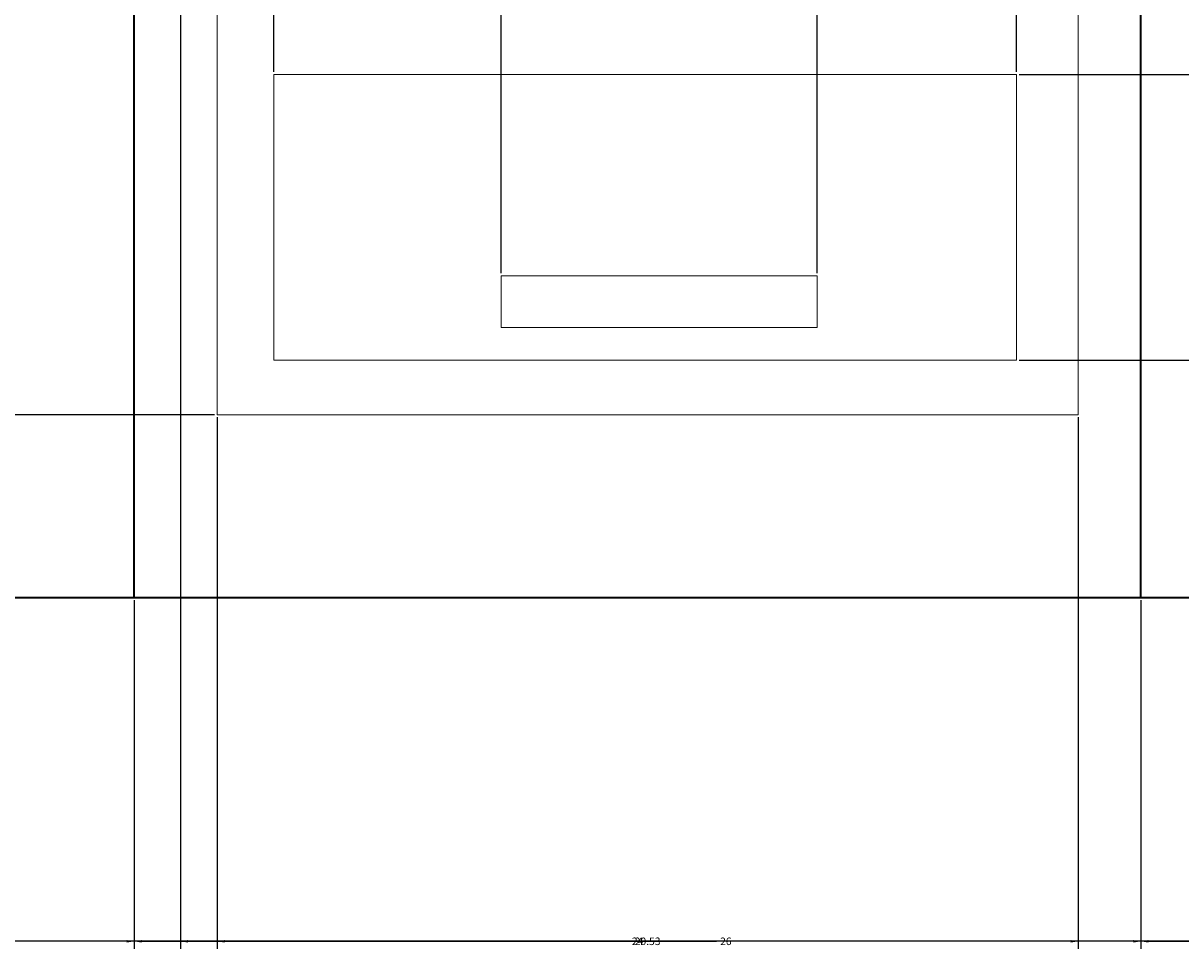
# Model space of a CAD drawing. Units: inches. Extents: x 27 to 200, y -50 to 102.
# Tile 10 of 26: x 117 to 144, y -25 to -3. Entities that reach past the tile are written whole.
import ezdxf

# ---------------------------------------------------------------- set-up
doc = ezdxf.new("R2010")
doc.units = ezdxf.units.IN
doc.header["$MEASUREMENT"] = 0
for name, color, linetype, lineweight in [('A-ANNO-DIMS', 2, 'Continuous', 18), ('A-ELEV', 7, 'Continuous', 35), ('A-FURN', 8, 'Continuous', 18)]:
    doc.layers.add(name, color=color, linetype=linetype, lineweight=lineweight)
doc.styles.get("Standard").update_dxf_attribs({"font": 'arial.ttf'})
doc.dimstyles.get("Standard").update_dxf_attribs({"dimtxt": 0.18, "dimasz": 0.18, "dimexe": 0.18, "dimexo": 0.0625, "dimgap": 0.09, "dimtad": 0, "dimtih": 1, "dimtoh": 1, "dimdec": 4, "dimzin": 0, "dimdsep": 46, "dimtxsty": 'Standard', "dimcen": 0.09, "dimadec": 0, "dimazin": 0, "dimtfac": 1, "dimtdec": 4, "dimtofl": 0, "dimtmove": 0, "dimatfit": 3, "dimfxl": 1, "dimtolj": 1, "dimtzin": 0, "dimarcsym": 0})

# ---------------------------------------------------------------- blocks, each defined once
blk = doc.blocks.new('*D23')
at = {"layer": 'A-ANNO-DIMS', "color": 0, "lineweight": -2, "transparency": 16777216}
for p, q in [((35.417, -16.832), (35.417, -25.149)), ((191.417, -16.832), (191.417, -25.149)), ((35.597, -24.969), (113.137, -24.969)), ((191.237, -24.969), (113.697, -24.969))]:
    blk.add_line(p, q, dxfattribs=at)
at = {"layer": 'A-ANNO-DIMS', "color": 0, "transparency": 16777216}
for points in [[(35.597, -24.939), (35.597, -24.999), (35.417, -24.969)], [(191.237, -24.939), (191.237, -24.999), (191.417, -24.969)]]:
    blk.add_solid(points, dxfattribs=at)
at = {"layer": 'Defpoints', "color": 0, "transparency": 16777216}
for p in [(35.417, -16.769), (191.417, -16.769), (191.417, -24.969)]:
    blk.add_point(p, dxfattribs=at)
at = {"layer": 'A-ANNO-DIMS', "color": 0, "transparency": 16777216, "insert": (113.417, -24.969), "char_height": 0.18, "attachment_point": 5}
blk.add_mtext('\\A1;156', dxfattribs=at)
blk = doc.blocks.new('*D36')
at = {"layer": 'A-ANNO-DIMS', "color": 0, "lineweight": -2, "transparency": 16777216}
for p, q in [((107.312, -16.832), (107.312, -25.149)), ((119.312, -16.832), (119.312, -25.149)), ((107.492, -24.969), (113.102, -24.969)), ((119.132, -24.969), (113.521, -24.969))]:
    blk.add_line(p, q, dxfattribs=at)
at = {"layer": 'A-ANNO-DIMS', "color": 0, "transparency": 16777216}
for points in [[(107.492, -24.939), (107.492, -24.999), (107.312, -24.969)], [(119.132, -24.939), (119.132, -24.999), (119.312, -24.969)]]:
    blk.add_solid(points, dxfattribs=at)
at = {"layer": 'Defpoints', "color": 0, "transparency": 16777216}
for p in [(107.312, -16.769), (119.312, -16.769), (119.312, -24.969)]:
    blk.add_point(p, dxfattribs=at)
at = {"layer": 'A-ANNO-DIMS', "color": 0, "transparency": 16777216, "insert": (113.312, -24.969), "char_height": 0.18, "attachment_point": 5}
blk.add_mtext('\\A1;12', dxfattribs=at)
blk = doc.blocks.new('*D37')
at = {"layer": 'A-ANNO-DIMS', "color": 0, "lineweight": -2, "transparency": 16777216}
for p, q in [((119.312, -16.832), (119.312, -25.149)), ((143.312, -16.832), (143.312, -25.149)), ((119.492, -24.969), (131.092, -24.969)), ((143.132, -24.969), (131.532, -24.969))]:
    blk.add_line(p, q, dxfattribs=at)
at = {"layer": 'A-ANNO-DIMS', "color": 0, "transparency": 16777216}
for points in [[(119.492, -24.939), (119.492, -24.999), (119.312, -24.969)], [(143.132, -24.939), (143.132, -24.999), (143.312, -24.969)]]:
    blk.add_solid(points, dxfattribs=at)
at = {"layer": 'Defpoints', "color": 0, "transparency": 16777216}
for p in [(119.312, -16.769), (143.312, -16.769), (143.312, -24.969)]:
    blk.add_point(p, dxfattribs=at)
at = {"layer": 'A-ANNO-DIMS', "color": 0, "transparency": 16777216, "insert": (131.312, -24.969), "char_height": 0.18, "attachment_point": 5}
blk.add_mtext('\\A1;24', dxfattribs=at)
blk = doc.blocks.new('*D38')
at = {"layer": 'A-ANNO-DIMS', "color": 0, "lineweight": -2, "transparency": 16777216}
for p, q in [((143.312, -16.832), (143.312, -25.149)), ((167.312, -16.832), (167.312, -25.149)), ((143.492, -24.969), (155.092, -24.969)), ((167.132, -24.969), (155.532, -24.969))]:
    blk.add_line(p, q, dxfattribs=at)
at = {"layer": 'A-ANNO-DIMS', "color": 0, "transparency": 16777216}
for points in [[(143.492, -24.939), (143.492, -24.999), (143.312, -24.969)], [(167.132, -24.939), (167.132, -24.999), (167.312, -24.969)]]:
    blk.add_solid(points, dxfattribs=at)
at = {"layer": 'Defpoints', "color": 0, "transparency": 16777216}
for p in [(143.312, -16.769), (167.312, -16.769), (167.312, -24.969)]:
    blk.add_point(p, dxfattribs=at)
at = {"layer": 'A-ANNO-DIMS', "color": 0, "transparency": 16777216, "insert": (155.312, -24.969), "char_height": 0.18, "attachment_point": 5}
blk.add_mtext('\\A1;24', dxfattribs=at)
blk = doc.blocks.new('*D48')
at = {"layer": 'A-ANNO-DIMS', "color": 0, "lineweight": -2, "transparency": 16777216}
for p, q in [((84.479, 44.926), (199.797, 44.926)), ((199.617, 44.746), (199.617, 14.26)), ((199.617, -16.589), (199.617, 13.897)), ((84.479, -16.769), (199.797, -16.769))]:
    blk.add_line(p, q, dxfattribs=at)
at = {"layer": 'A-ANNO-DIMS', "color": 0, "transparency": 16777216}
for points in [[(199.587, 44.746), (199.647, 44.746), (199.617, 44.926)], [(199.587, -16.589), (199.647, -16.589), (199.617, -16.769)]]:
    blk.add_solid(points, dxfattribs=at)
at = {"layer": 'Defpoints', "color": 0, "transparency": 16777216}
for p in [(84.417, 44.926), (199.617, 44.926), (84.417, -16.769)]:
    blk.add_point(p, dxfattribs=at)
at = {"layer": 'A-ANNO-DIMS', "color": 0, "transparency": 16777216, "insert": (199.617, 14.079), "char_height": 0.18, "attachment_point": 5}
blk.add_mtext('\\A1;61.7', dxfattribs=at)
blk = doc.blocks.new('*D51')
at = {"layer": 'A-ANNO-DIMS', "color": 0, "lineweight": -2, "transparency": 16777216}
for p, q in [((120.417, 45.561), (120.417, -25.149)), ((146.417, 45.561), (146.417, -25.149)), ((120.597, -24.969), (133.197, -24.969)), ((146.237, -24.969), (133.637, -24.969))]:
    blk.add_line(p, q, dxfattribs=at)
at = {"layer": 'A-ANNO-DIMS', "color": 0, "transparency": 16777216}
for points in [[(120.597, -24.939), (120.597, -24.999), (120.417, -24.969)], [(146.237, -24.939), (146.237, -24.999), (146.417, -24.969)]]:
    blk.add_solid(points, dxfattribs=at)
at = {"layer": 'Defpoints', "color": 0, "transparency": 16777216}
for p in [(120.417, 45.623), (146.417, 45.623), (146.417, -24.969)]:
    blk.add_point(p, dxfattribs=at)
at = {"layer": 'A-ANNO-DIMS', "color": 0, "transparency": 16777216, "insert": (133.417, -24.969), "char_height": 0.18, "attachment_point": 5}
blk.add_mtext('\\A1;26', dxfattribs=at)
blk = doc.blocks.new('*D55')
at = {"layer": 'A-ANNO-DIMS', "color": 0, "lineweight": -2, "transparency": 16777216}
for p, q in [((121.288, -12.473), (121.288, -25.149)), ((141.816, -12.473), (141.816, -25.149)), ((121.468, -24.969), (131.157, -24.969)), ((141.636, -24.969), (131.947, -24.969))]:
    blk.add_line(p, q, dxfattribs=at)
at = {"layer": 'A-ANNO-DIMS', "color": 0, "transparency": 16777216}
for points in [[(121.468, -24.939), (121.468, -24.999), (121.288, -24.969)], [(141.636, -24.939), (141.636, -24.999), (141.816, -24.969)]]:
    blk.add_solid(points, dxfattribs=at)
at = {"layer": 'Defpoints', "color": 0, "transparency": 16777216}
for p in [(121.288, -12.411), (141.816, -12.411), (141.816, -24.969)]:
    blk.add_point(p, dxfattribs=at)
at = {"layer": 'A-ANNO-DIMS', "color": 0, "transparency": 16777216, "insert": (131.552, -24.969), "char_height": 0.18, "attachment_point": 5}
blk.add_mtext('\\A1;20.53', dxfattribs=at)
blk = doc.blocks.new('*D56')
at = {"layer": 'A-ANNO-DIMS', "color": 0, "lineweight": -2, "transparency": 16777216}
for p, q in [((121.225, 5.878), (27.037, 5.878)), ((27.217, 5.698), (27.217, -3.085)), ((27.217, -12.231), (27.217, -3.448)), ((121.225, -12.411), (27.037, -12.411))]:
    blk.add_line(p, q, dxfattribs=at)
at = {"layer": 'A-ANNO-DIMS', "color": 0, "transparency": 16777216}
for points in [[(27.187, 5.698), (27.247, 5.698), (27.217, 5.878)], [(27.187, -12.231), (27.247, -12.231), (27.217, -12.411)]]:
    blk.add_solid(points, dxfattribs=at)
at = {"layer": 'Defpoints', "color": 0, "transparency": 16777216}
for p in [(27.217, 5.878), (121.288, 5.878), (121.288, -12.411)]:
    blk.add_point(p, dxfattribs=at)
at = {"layer": 'A-ANNO-DIMS', "color": 0, "transparency": 16777216, "insert": (27.217, -3.267), "char_height": 0.18, "attachment_point": 5}
blk.add_mtext('\\A1;18.29', dxfattribs=at)
blk = doc.blocks.new('*D61')
at = {"layer": 'A-ANNO-DIMS', "color": 0, "lineweight": -2, "transparency": 16777216}
for p, q in [((122.638, -4.237), (122.638, 102.306)), ((122.818, 102.126), (131.125, 102.126)), ((140.167, 102.126), (131.86, 102.126)), ((140.347, -4.237), (140.347, 102.306))]:
    blk.add_line(p, q, dxfattribs=at)
at = {"layer": 'A-ANNO-DIMS', "color": 0, "transparency": 16777216}
for points in [[(122.818, 102.156), (122.818, 102.096), (122.638, 102.126)], [(140.167, 102.156), (140.167, 102.096), (140.347, 102.126)]]:
    blk.add_solid(points, dxfattribs=at)
at = {"layer": 'Defpoints', "color": 0, "transparency": 16777216}
for p in [(140.347, 102.126), (122.638, -4.3), (140.347, -4.3)]:
    blk.add_point(p, dxfattribs=at)
at = {"layer": 'A-ANNO-DIMS', "color": 0, "transparency": 16777216, "insert": (131.493, 102.126), "char_height": 0.18, "attachment_point": 5}
blk.add_mtext('\\A1;17.71', dxfattribs=at)
blk = doc.blocks.new('*D62')
at = {"layer": 'A-ANNO-DIMS', "color": 0, "lineweight": -2, "transparency": 16777216}
for p, q in [((140.41, -4.3), (199.797, -4.3)), ((199.617, -4.48), (199.617, -7.522)), ((199.617, -10.928), (199.617, -7.886)), ((140.41, -11.108), (199.797, -11.108))]:
    blk.add_line(p, q, dxfattribs=at)
at = {"layer": 'A-ANNO-DIMS', "color": 0, "transparency": 16777216}
for points in [[(199.587, -4.48), (199.647, -4.48), (199.617, -4.3)], [(199.587, -10.928), (199.647, -10.928), (199.617, -11.108)]]:
    blk.add_solid(points, dxfattribs=at)
at = {"layer": 'Defpoints', "color": 0, "transparency": 16777216}
for p in [(140.347, -4.3), (199.617, -4.3), (140.347, -11.108)]:
    blk.add_point(p, dxfattribs=at)
at = {"layer": 'A-ANNO-DIMS', "color": 0, "transparency": 16777216, "insert": (199.617, -7.704), "char_height": 0.18, "attachment_point": 5}
blk.add_mtext('\\A1;6.809', dxfattribs=at)
blk = doc.blocks.new('*D63')
at = {"layer": 'A-ANNO-DIMS', "color": 0, "lineweight": -2, "transparency": 16777216}
for p, q in [((128.059, -9.034), (128.059, 102.306)), ((128.239, 102.126), (131.435, 102.126)), ((135.417, 102.126), (132.221, 102.126)), ((135.597, -9.034), (135.597, 102.306))]:
    blk.add_line(p, q, dxfattribs=at)
at = {"layer": 'A-ANNO-DIMS', "color": 0, "transparency": 16777216}
for points in [[(128.239, 102.156), (128.239, 102.096), (128.059, 102.126)], [(135.417, 102.156), (135.417, 102.096), (135.597, 102.126)]]:
    blk.add_solid(points, dxfattribs=at)
at = {"layer": 'Defpoints', "color": 0, "transparency": 16777216}
for p in [(135.597, 102.126), (128.059, -9.097), (135.597, -9.097)]:
    blk.add_point(p, dxfattribs=at)
at = {"layer": 'A-ANNO-DIMS', "color": 0, "transparency": 16777216, "insert": (131.828, 102.126), "char_height": 0.18, "attachment_point": 5}
blk.add_mtext('\\A1;7.538', dxfattribs=at)
blk = doc.blocks.new('*D69')
at = {"layer": 'A-ANNO-DIMS', "color": 0, "lineweight": -2, "transparency": 16777216}
for p, q in [((121.225, -12.411), (27.037, -12.411)), ((27.217, -12.591), (27.217, -14.408)), ((27.217, -16.589), (27.217, -14.772)), ((119.249, -16.769), (27.037, -16.769))]:
    blk.add_line(p, q, dxfattribs=at)
at = {"layer": 'A-ANNO-DIMS', "color": 0, "transparency": 16777216}
for points in [[(27.187, -12.591), (27.247, -12.591), (27.217, -12.411)], [(27.187, -16.589), (27.247, -16.589), (27.217, -16.769)]]:
    blk.add_solid(points, dxfattribs=at)
at = {"layer": 'Defpoints', "color": 0, "transparency": 16777216}
for p in [(27.217, -12.411), (121.288, -12.411), (119.312, -16.769)]:
    blk.add_point(p, dxfattribs=at)
at = {"layer": 'A-ANNO-DIMS', "color": 0, "transparency": 16777216, "insert": (27.217, -14.59), "char_height": 0.18, "attachment_point": 5}
blk.add_mtext('\\A1;4.358', dxfattribs=at)

msp = doc.modelspace()

# ---------------------------------------------------------------- linework, layer by layer
at = {"layer": 'A-ELEV'}
for p, q in [((119.3118, -16.7693), (119.3118, 16.1635)), ((143.3118, -16.7693), (143.3118, 16.1097)), ((35.4169, -16.7693), (191.4169, -16.7693))]:
    msp.add_line(p, q, dxfattribs=at)
at = {"layer": 'A-FURN'}
for points in [[(121.2876, 5.8779), (141.8163, 5.8779), (141.8163, -12.411), (121.2876, -12.411)], [(122.6381, -4.2997), (140.3471, -4.2997), (140.3471, -11.1085), (122.6381, -11.1085)], [(128.0592, -9.0968), (135.5972, -9.0968), (135.5972, -10.3348), (128.0592, -10.3348)]]:
    msp.add_lwpolyline(points, close=True, dxfattribs=at)

# ---------------------------------------------------------------- dimensions: what is measured, and where the dimension line sits
at = {"layer": 'A-ANNO-DIMS'}
for base, p1, p2, override, picture, middle in [((140.3471, 102.1264), (122.6381, -4.2997), (140.3471, -4.2997), {"dimdec": 2, "dimlfac": 1, "dimrnd": 0, "dimzin": 0, "dimdsep": 46, "dimlunit": 2}, '*D61', (131.4926, 102.1264)), ((135.5972, 102.1264), (128.0592, -9.0968), (135.5972, -9.0968), {"dimdec": 3, "dimlfac": 1, "dimrnd": 0, "dimzin": 0, "dimdsep": 46, "dimlunit": 2}, '*D63', (131.8282, 102.1264)), ((146.4169, -24.9693), (120.4169, 45.6231), (146.4169, 45.6231), {"dimdec": 0, "dimlfac": 1, "dimrnd": 0, "dimzin": 0, "dimdsep": 46, "dimlunit": 2}, '*D51', (133.4169, -24.9693)), ((141.8163, -24.9693), (121.2876, -12.411), (141.8163, -12.411), {"dimdec": 2, "dimlfac": 1, "dimrnd": 0, "dimzin": 0, "dimdsep": 46, "dimlunit": 2}, '*D55', (131.552, -24.9693)), ((191.4169, -24.9693), (35.4169, -16.7693), (191.4169, -16.7693), {"dimdec": 0, "dimlfac": 1, "dimrnd": 0, "dimzin": 0, "dimdsep": 46, "dimlunit": 2}, '*D23', (113.4169, -24.9693)), ((119.3118, -24.9693), (107.3118, -16.7693), (119.3118, -16.7693), {"dimdec": 0, "dimlfac": 1, "dimrnd": 0, "dimzin": 0, "dimdsep": 46, "dimlunit": 2}, '*D36', (113.3118, -24.9693)), ((143.3118, -24.9693), (119.3118, -16.7693), (143.3118, -16.7693), {"dimdec": 0, "dimlfac": 1, "dimrnd": 0, "dimzin": 0, "dimdsep": 46, "dimlunit": 2}, '*D37', (131.3118, -24.9693)), ((167.3118, -24.9693), (143.3118, -16.7693), (167.3118, -16.7693), {"dimdec": 0, "dimlfac": 1, "dimrnd": 0, "dimzin": 0, "dimdsep": 46, "dimlunit": 2}, '*D38', (155.3118, -24.9693))]:
    dim = msp.add_linear_dim(base=base, p1=p1, p2=p2, dimstyle='Standard', override=override, dxfattribs=at)
    dim.commit()
    dim.dimension.update_dxf_attribs({"geometry": picture, "text_midpoint": middle})
for base, p1, p2, override, picture, middle in [((199.6169, 44.9264), (84.4169, -16.7693), (84.4169, 44.9264), {"dimdec": 1, "dimlfac": 1, "dimrnd": 0, "dimzin": 0, "dimdsep": 46, "dimlunit": 2}, '*D48', (199.6169, 14.0786)), ((27.2169, 5.8779), (121.2876, -12.411), (121.2876, 5.8779), {"dimdec": 2, "dimlfac": 1, "dimrnd": 0, "dimzin": 0, "dimdsep": 46, "dimlunit": 2}, '*D56', (27.2169, -3.2665)), ((199.6169, -4.2997), (140.3471, -11.1085), (140.3471, -4.2997), {"dimdec": 3, "dimlfac": 1, "dimrnd": 0, "dimzin": 0, "dimdsep": 46, "dimlunit": 2}, '*D62', (199.6169, -7.7041)), ((27.2169, -12.411), (119.3118, -16.7693), (121.2876, -12.411), {"dimdec": 3, "dimlfac": 1, "dimrnd": 0, "dimzin": 0, "dimdsep": 46, "dimlunit": 2}, '*D69', (27.2169, -14.5901))]:
    dim = msp.add_linear_dim(base=base, p1=p1, p2=p2, angle=90, dimstyle='Standard', override=override, dxfattribs=at)
    dim.commit()
    dim.dimension.update_dxf_attribs({"geometry": picture, "text_midpoint": middle})

doc.saveas('drawing.dxf')
